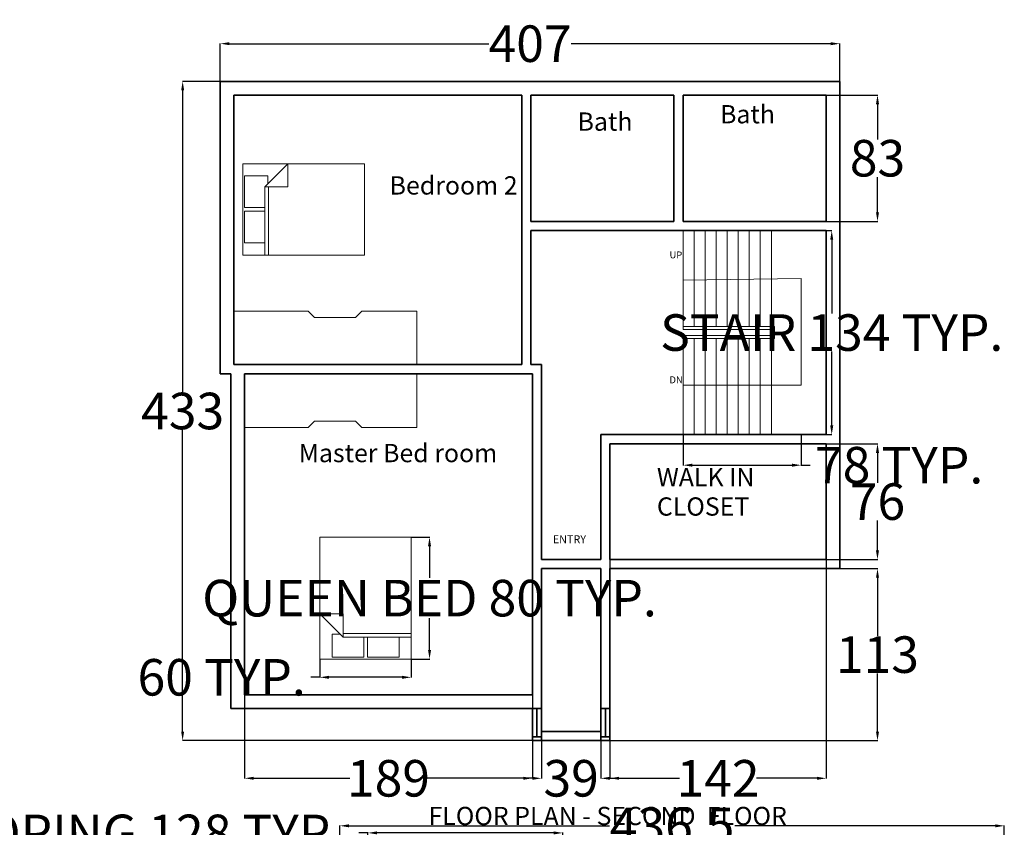
# Model space of a CAD drawing. Units: inches. Extents: x -15 to 1815, y 1023 to 2303.
# Tile 8 of 8: x 910 to 1556, y 1773 to 2303. Entities that reach past the tile are written whole.
import ezdxf

# ---------------------------------------------------------------- set-up
doc = ezdxf.new("R2010")
doc.units = ezdxf.units.IN
doc.header["$MEASUREMENT"] = 0
for name, color, linetype, lineweight in [('A-ANNO-DIMS', 2, 'Continuous', 18), ('A-ANNO-TEXT', 7, 'Continuous', 25), ('A-AREA-IDEN', 7, 'Continuous', 18), ('A-FLOR-STRS', 3, 'Continuous', 18), ('A-FURN', 8, 'Continuous', 18), ('A-WALL', 7, 'Continuous', 35)]:
    doc.layers.add(name, color=color, linetype=linetype, lineweight=lineweight)
doc.styles.get("Standard").update_dxf_attribs({"font": 'arial.ttf'})
doc.dimstyles.get("Standard").update_dxf_attribs({"dimtxt": 24, "dimasz": 6, "dimexe": 0.18, "dimexo": 0.0625, "dimgap": 0.09, "dimtad": 0, "dimtih": 1, "dimtoh": 1, "dimdec": 0, "dimzin": 0, "dimdsep": 46, "dimlunit": 3, "dimtxsty": 'Standard', "dimcen": 0.09, "dimadec": 0, "dimazin": 0, "dimtfac": 1, "dimtdec": 0, "dimtofl": 0, "dimtmove": 0, "dimatfit": 3, "dimfxl": 1, "dimtolj": 1, "dimtzin": 0, "dimarcsym": 0})

# ---------------------------------------------------------------- blocks, each defined once
blk = doc.blocks.new('Bed - Queen')
for p, q in [((0, -80.00003), (0, 0)), ((0, 0), (59.99999, 0)), ((59.99999, 0), (59.99999, -80.00003)), ((7.99999, -1.2), (28.79998, -1.2)), ((7.99999, -14.4), (7.99999, -1.2)), ((28.79998, -1.2), (28.79998, -14.4)), ((31.19999, -1.2), (51.99999, -1.2)), ((31.19999, -14.4), (31.19999, -1.2)), ((51.99999, -1.2), (51.99999, -16.4)), ((0, -14.4), (44.8, -14.4)), ((44.8, -16.8), (0, -16.8)), ((59.99999, -29.6), (44.8, -14.4)), ((44.8, -14.4), (44.8, -29.6)), ((51.99999, -16.4), (46.79936, -16.4)), ((44.8, -29.6), (59.99999, -29.6)), ((59.99999, -80.00003), (0, -80.00003))]:
    blk.add_line(p, q)
blk = doc.blocks.new('STAIR-RETURN-PLAN')
for p, q in [((0, 69), (0, 134)), ((7.25, 71), (7.25, 134)), ((14.5, 71), (14.5, 134)), ((21.75, 71), (21.75, 134)), ((29, 71), (29, 134)), ((36.25, 71), (36.25, 134)), ((43.5, 71), (43.5, 134)), ((50.75, 71), (50.75, 134)), ((58, 71), (58, 134)), ((58, 71), (58, 134)), ((0, 101.5), (77.56, 102.5)), ((77.56, 102.5), (77.56, 32.54)), ((60, 71), (0, 71)), ((58, 69), (0, 69)), ((58, 65), (0, 65)), ((0, 0), (0, 65)), ((58, 65), (58, 69)), ((60, 65), (60, 71)), ((60, 63), (60, 65)), ((60, 63), (0, 63)), ((7.25, 0), (7.25, 63)), ((14.5, 0), (14.5, 63)), ((21.75, 0), (21.75, 63)), ((29, 0), (29, 63)), ((36.25, 0), (36.25, 63)), ((43.5, 0), (43.5, 63)), ((50.75, 0), (50.75, 63)), ((58, 0), (58, 63)), ((58, 0), (58, 63)), ((77.56, 32.54), (0, 32.5))]:
    blk.add_line(p, q)
blk = doc.blocks.new('*D23')
at = {"layer": 'A-ANNO-DIMS', "color": 0, "lineweight": -2, "transparency": 16777216}
for p, q in [((1166.94, 1963.35), (1179.06, 1963.35)), ((1178.88, 1957.35), (1178.88, 1936.58)), ((1178.88, 1889.35), (1178.88, 1910.11)), ((1166.94, 1883.35), (1179.06, 1883.35))]:
    blk.add_line(p, q, dxfattribs=at)
at = {"layer": 'A-ANNO-DIMS', "color": 0, "transparency": 16777216}
for points in [[(1177.88, 1957.35), (1179.88, 1957.35), (1178.88, 1963.35)], [(1177.88, 1889.35), (1179.88, 1889.35), (1178.88, 1883.35)]]:
    blk.add_solid(points, dxfattribs=at)
at = {"layer": 'Defpoints', "color": 0, "transparency": 16777216}
for p in [(1166.88, 1963.35), (1166.88, 1883.35), (1178.88, 1883.35)]:
    blk.add_point(p, dxfattribs=at)
at = {"layer": 'A-ANNO-DIMS', "color": 0, "transparency": 16777216, "insert": (1178.88, 1923.35), "char_height": 24, "attachment_point": 5}
blk.add_mtext('\\A1;QUEEN BED 80 TYP.', dxfattribs=at)
blk = doc.blocks.new('*D24')
at = {"layer": 'A-ANNO-DIMS', "color": 0, "lineweight": -2, "transparency": 16777216}
for p, q in [((1106.88, 1883.29), (1106.88, 1871.17)), ((1166.88, 1883.29), (1166.88, 1871.17)), ((1106.88, 1871.35), (1100.88, 1871.35)), ((1160.88, 1871.35), (1112.88, 1871.35))]:
    blk.add_line(p, q, dxfattribs=at)
at = {"layer": 'A-ANNO-DIMS', "color": 0, "transparency": 16777216}
for points in [[(1112.88, 1872.35), (1112.88, 1870.35), (1106.88, 1871.35)], [(1160.88, 1872.35), (1160.88, 1870.35), (1166.88, 1871.35)]]:
    blk.add_solid(points, dxfattribs=at)
at = {"layer": 'Defpoints', "color": 0, "transparency": 16777216}
for p in [(1106.88, 1883.35), (1166.88, 1883.35), (1106.88, 1871.35)]:
    blk.add_point(p, dxfattribs=at)
at = {"layer": 'A-ANNO-DIMS', "color": 0, "transparency": 16777216, "insert": (1042.31, 1871.35), "char_height": 24, "attachment_point": 5}
blk.add_mtext('\\A1;60 TYP.', dxfattribs=at)
blk = doc.blocks.new('*D25')
at = {"layer": 'A-ANNO-DIMS', "color": 0, "lineweight": -2, "transparency": 16777216}
for p, q in [((1423.04, 2164.75), (1443.26, 2164.75)), ((1443.08, 2158.75), (1443.08, 2110.26)), ((1443.08, 2036.75), (1443.08, 2085.24)), ((1423.04, 2030.75), (1443.26, 2030.75))]:
    blk.add_line(p, q, dxfattribs=at)
at = {"layer": 'A-ANNO-DIMS', "color": 0, "transparency": 16777216}
for points in [[(1442.08, 2158.75), (1444.08, 2158.75), (1443.08, 2164.75)], [(1442.08, 2036.75), (1444.08, 2036.75), (1443.08, 2030.75)]]:
    blk.add_solid(points, dxfattribs=at)
at = {"layer": 'Defpoints', "color": 0, "transparency": 16777216}
for p in [(1422.98, 2164.75), (1443.08, 2164.75), (1422.98, 2030.75)]:
    blk.add_point(p, dxfattribs=at)
at = {"layer": 'A-ANNO-DIMS', "color": 0, "transparency": 16777216, "insert": (1443.08, 2097.75), "char_height": 24, "attachment_point": 5}
blk.add_mtext('\\A1;STAIR 134 TYP.', dxfattribs=at)
blk = doc.blocks.new('*D26')
at = {"layer": 'A-ANNO-DIMS', "color": 0, "lineweight": -2, "transparency": 16777216}
for p, q in [((1345.42, 2030.69), (1345.42, 2010.47)), ((1422.98, 2030.69), (1422.98, 2010.47)), ((1351.42, 2010.65), (1416.98, 2010.65)), ((1422.98, 2010.65), (1428.98, 2010.65))]:
    blk.add_line(p, q, dxfattribs=at)
at = {"layer": 'A-ANNO-DIMS', "color": 0, "transparency": 16777216}
for points in [[(1351.42, 2011.65), (1351.42, 2009.65), (1345.42, 2010.65)], [(1416.98, 2011.65), (1416.98, 2009.65), (1422.98, 2010.65)]]:
    blk.add_solid(points, dxfattribs=at)
at = {"layer": 'Defpoints', "color": 0, "transparency": 16777216}
for p in [(1345.42, 2030.75), (1422.98, 2030.75), (1422.98, 2010.65)]:
    blk.add_point(p, dxfattribs=at)
at = {"layer": 'A-ANNO-DIMS', "color": 0, "transparency": 16777216, "insert": (1487.38, 2010.65), "char_height": 24, "attachment_point": 5}
blk.add_mtext('\\A1;78 TYP.', dxfattribs=at)
blk = doc.blocks.new('*D45')
at = {"layer": 'A-ANNO-DIMS', "color": 0, "lineweight": -2, "transparency": 16777216}
for p, q in [((1138.43, 1769.16), (1132.43, 1769.16)), ((1138.43, 1750.02), (1138.43, 1769.34)), ((1260.44, 1769.16), (1144.43, 1769.16)), ((1266.44, 1750.02), (1266.44, 1769.34))]:
    blk.add_line(p, q, dxfattribs=at)
at = {"layer": 'A-ANNO-DIMS', "color": 0, "transparency": 16777216}
for points in [[(1144.43, 1770.16), (1144.43, 1768.16), (1138.43, 1769.16)], [(1260.44, 1770.16), (1260.44, 1768.16), (1266.44, 1769.16)]]:
    blk.add_solid(points, dxfattribs=at)
at = {"layer": 'Defpoints', "color": 0, "transparency": 16777216}
for p in [(1138.43, 1769.16), (1138.43, 1749.96), (1266.44, 1749.96)]:
    blk.add_point(p, dxfattribs=at)
at = {"layer": 'A-ANNO-DIMS', "color": 0, "transparency": 16777216, "insert": (993.96, 1769.16), "char_height": 24, "attachment_point": 5}
blk.add_mtext('\\A1;COPING 128 TYP.', dxfattribs=at)
blk = doc.blocks.new('*D80')
at = {"layer": 'A-ANNO-DIMS', "color": 0, "lineweight": -2, "transparency": 16777216}
for p, q in [((1041.42, 2262.81), (1041.42, 2287.66)), ((1047.42, 2287.48), (1217.83, 2287.48)), ((1442.42, 2287.48), (1272, 2287.48)), ((1448.42, 2262.81), (1448.42, 2287.66))]:
    blk.add_line(p, q, dxfattribs=at)
at = {"layer": 'A-ANNO-DIMS', "color": 0, "transparency": 16777216}
for points in [[(1047.42, 2288.48), (1047.42, 2286.48), (1041.42, 2287.48)], [(1442.42, 2288.48), (1442.42, 2286.48), (1448.42, 2287.48)]]:
    blk.add_solid(points, dxfattribs=at)
at = {"layer": 'Defpoints', "color": 0, "transparency": 16777216}
for p in [(1448.42, 2287.48), (1041.42, 2262.75), (1448.42, 2262.75)]:
    blk.add_point(p, dxfattribs=at)
at = {"layer": 'A-ANNO-DIMS', "color": 0, "transparency": 16777216, "insert": (1244.92, 2287.48), "char_height": 24, "attachment_point": 5}
blk.add_mtext('\\A1;407', dxfattribs=at)
blk = doc.blocks.new('*D81')
at = {"layer": 'A-ANNO-DIMS', "color": 0, "lineweight": -2, "transparency": 16777216}
for p, q in [((1041.36, 2262.75), (1016.51, 2262.75)), ((1016.69, 2256.75), (1016.69, 2058.6)), ((1016.69, 1835.75), (1016.69, 2033.9)), ((1246.36, 1829.75), (1016.51, 1829.75))]:
    blk.add_line(p, q, dxfattribs=at)
at = {"layer": 'A-ANNO-DIMS', "color": 0, "transparency": 16777216}
for points in [[(1015.69, 2256.75), (1017.69, 2256.75), (1016.69, 2262.75)], [(1015.69, 1835.75), (1017.69, 1835.75), (1016.69, 1829.75)]]:
    blk.add_solid(points, dxfattribs=at)
at = {"layer": 'Defpoints', "color": 0, "transparency": 16777216}
for p in [(1041.42, 2262.75), (1016.69, 1829.75), (1246.42, 1829.75)]:
    blk.add_point(p, dxfattribs=at)
at = {"layer": 'A-ANNO-DIMS', "color": 0, "transparency": 16777216, "insert": (1016.69, 2046.25), "char_height": 24, "attachment_point": 5}
blk.add_mtext('\\A1;433', dxfattribs=at)
blk = doc.blocks.new('*D82')
at = {"layer": 'A-ANNO-DIMS', "color": 0, "lineweight": -2, "transparency": 16777216}
for p, q in [((1448.48, 1942.75), (1473.33, 1942.75)), ((1473.15, 1936.75), (1473.15, 1898.6)), ((1473.15, 1835.75), (1473.15, 1873.9)), ((1297.48, 1829.75), (1473.33, 1829.75))]:
    blk.add_line(p, q, dxfattribs=at)
at = {"layer": 'A-ANNO-DIMS', "color": 0, "transparency": 16777216}
for points in [[(1472.15, 1936.75), (1474.15, 1936.75), (1473.15, 1942.75)], [(1472.15, 1835.75), (1474.15, 1835.75), (1473.15, 1829.75)]]:
    blk.add_solid(points, dxfattribs=at)
at = {"layer": 'Defpoints', "color": 0, "transparency": 16777216}
for p in [(1448.42, 1942.75), (1473.15, 1942.75), (1297.42, 1829.75)]:
    blk.add_point(p, dxfattribs=at)
at = {"layer": 'A-ANNO-DIMS', "color": 0, "transparency": 16777216, "insert": (1473.15, 1886.25), "char_height": 24, "attachment_point": 5}
blk.add_mtext('\\A1;113', dxfattribs=at)
blk = doc.blocks.new('*D83')
at = {"layer": 'A-ANNO-DIMS', "color": 0, "lineweight": -2, "transparency": 16777216}
for p, q in [((1439.48, 2024.75), (1473.33, 2024.75)), ((1473.15, 2018.75), (1473.15, 1999.09)), ((1473.15, 1954.75), (1473.15, 1974.41)), ((1439.48, 1948.75), (1473.33, 1948.75))]:
    blk.add_line(p, q, dxfattribs=at)
at = {"layer": 'A-ANNO-DIMS', "color": 0, "transparency": 16777216}
for points in [[(1472.15, 2018.75), (1474.15, 2018.75), (1473.15, 2024.75)], [(1472.15, 1954.75), (1474.15, 1954.75), (1473.15, 1948.75)]]:
    blk.add_solid(points, dxfattribs=at)
at = {"layer": 'Defpoints', "color": 0, "transparency": 16777216}
for p in [(1439.42, 2024.75), (1473.15, 2024.75), (1439.42, 1948.75)]:
    blk.add_point(p, dxfattribs=at)
at = {"layer": 'A-ANNO-DIMS', "color": 0, "transparency": 16777216, "insert": (1473.15, 1986.75), "char_height": 24, "attachment_point": 5}
blk.add_mtext('\\A1;76', dxfattribs=at)
blk = doc.blocks.new('*D84')
at = {"layer": 'A-ANNO-DIMS', "color": 0, "lineweight": -2, "transparency": 16777216}
for p, q in [((1439.48, 2253.75), (1473.33, 2253.75)), ((1473.15, 2247.75), (1473.15, 2224.6)), ((1473.15, 2176.75), (1473.15, 2199.9)), ((1439.48, 2170.75), (1473.33, 2170.75))]:
    blk.add_line(p, q, dxfattribs=at)
at = {"layer": 'A-ANNO-DIMS', "color": 0, "transparency": 16777216}
for points in [[(1472.15, 2247.75), (1474.15, 2247.75), (1473.15, 2253.75)], [(1472.15, 2176.75), (1474.15, 2176.75), (1473.15, 2170.75)]]:
    blk.add_solid(points, dxfattribs=at)
at = {"layer": 'Defpoints', "color": 0, "transparency": 16777216}
for p in [(1439.42, 2253.75), (1473.15, 2253.75), (1439.42, 2170.75)]:
    blk.add_point(p, dxfattribs=at)
at = {"layer": 'A-ANNO-DIMS', "color": 0, "transparency": 16777216, "insert": (1473.15, 2212.25), "char_height": 24, "attachment_point": 5}
blk.add_mtext('\\A1;83', dxfattribs=at)
blk = doc.blocks.new('*D85')
at = {"layer": 'A-ANNO-DIMS', "color": 0, "lineweight": -2, "transparency": 16777216}
for p, q in [((1057.42, 1859.69), (1057.42, 1804.84)), ((1246.42, 1859.69), (1246.42, 1804.84)), ((1063.42, 1805.02), (1126.42, 1805.02)), ((1240.42, 1805.02), (1177.42, 1805.02))]:
    blk.add_line(p, q, dxfattribs=at)
at = {"layer": 'A-ANNO-DIMS', "color": 0, "transparency": 16777216}
for points in [[(1063.42, 1806.02), (1063.42, 1804.02), (1057.42, 1805.02)], [(1240.42, 1806.02), (1240.42, 1804.02), (1246.42, 1805.02)]]:
    blk.add_solid(points, dxfattribs=at)
at = {"layer": 'Defpoints', "color": 0, "transparency": 16777216}
for p in [(1057.42, 1859.75), (1246.42, 1859.75), (1246.42, 1805.02)]:
    blk.add_point(p, dxfattribs=at)
at = {"layer": 'A-ANNO-DIMS', "color": 0, "transparency": 16777216, "insert": (1151.92, 1805.02), "char_height": 24, "attachment_point": 5}
blk.add_mtext('\\A1;189', dxfattribs=at)
blk = doc.blocks.new('*D86')
at = {"layer": 'A-ANNO-DIMS', "color": 0, "lineweight": -2, "transparency": 16777216}
for p, q in [((1252.417621, 1850.68843), (1252.417621, 1804.83843)), ((1291.417621, 1850.68843), (1291.417621, 1804.83843)), ((1246.417621, 1805.01843), (1240.417621, 1805.01843)), ((1297.417621, 1805.01843), (1303.417621, 1805.01843))]:
    blk.add_line(p, q, dxfattribs=at)
at = {"layer": 'A-ANNO-DIMS', "color": 0, "transparency": 16777216}
for points in [[(1246.417621, 1806.01843), (1246.417621, 1804.01843), (1252.417621, 1805.01843)], [(1297.417621, 1806.01843), (1297.417621, 1804.01843), (1291.417621, 1805.01843)]]:
    blk.add_solid(points, dxfattribs=at)
at = {"layer": 'Defpoints', "color": 0, "transparency": 16777216}
for p in [(1252.417621, 1850.75093), (1291.417621, 1850.75093), (1291.417621, 1805.01843)]:
    blk.add_point(p, dxfattribs=at)
at = {"layer": 'A-ANNO-DIMS', "color": 0, "transparency": 16777216, "insert": (1271.917621, 1805.01843), "char_height": 24, "attachment_point": 5}
blk.add_mtext('\\A1;39', dxfattribs=at)
blk = doc.blocks.new('*D87')
at = {"layer": 'A-ANNO-DIMS', "color": 0, "lineweight": -2, "transparency": 16777216}
for p, q in [((1297.42, 1948.69), (1297.42, 1804.84)), ((1439.42, 1948.69), (1439.42, 1804.84)), ((1303.42, 1805.02), (1343.07, 1805.02)), ((1433.42, 1805.02), (1393.77, 1805.02))]:
    blk.add_line(p, q, dxfattribs=at)
at = {"layer": 'A-ANNO-DIMS', "color": 0, "transparency": 16777216}
for points in [[(1303.42, 1806.02), (1303.42, 1804.02), (1297.42, 1805.02)], [(1433.42, 1806.02), (1433.42, 1804.02), (1439.42, 1805.02)]]:
    blk.add_solid(points, dxfattribs=at)
at = {"layer": 'Defpoints', "color": 0, "transparency": 16777216}
for p in [(1297.42, 1948.75), (1439.42, 1948.75), (1439.42, 1805.02)]:
    blk.add_point(p, dxfattribs=at)
at = {"layer": 'A-ANNO-DIMS', "color": 0, "transparency": 16777216, "insert": (1368.42, 1805.02), "char_height": 24, "attachment_point": 5}
blk.add_mtext('\\A1;142', dxfattribs=at)
blk = doc.blocks.new('*D103')
at = {"layer": 'A-ANNO-DIMS', "color": 0, "lineweight": -2, "transparency": 16777216}
for p, q in [((1119.96, 1657.14), (1119.96, 1773.99)), ((1125.96, 1773.81), (1297.05, 1773.81)), ((1550.46, 1773.81), (1379.37, 1773.81)), ((1556.46, 1657.14), (1556.46, 1773.99))]:
    blk.add_line(p, q, dxfattribs=at)
at = {"layer": 'A-ANNO-DIMS', "color": 0, "transparency": 16777216}
for points in [[(1125.96, 1774.81), (1125.96, 1772.81), (1119.96, 1773.81)], [(1550.46, 1774.81), (1550.46, 1772.81), (1556.46, 1773.81)]]:
    blk.add_solid(points, dxfattribs=at)
at = {"layer": 'Defpoints', "color": 0, "transparency": 16777216}
for p in [(1556.46, 1773.81), (1119.96, 1657.08), (1556.46, 1657.08)]:
    blk.add_point(p, dxfattribs=at)
at = {"layer": 'A-ANNO-DIMS', "color": 0, "transparency": 16777216, "insert": (1338.21, 1773.81), "char_height": 24, "attachment_point": 5}
blk.add_mtext('\\A1;436.5', dxfattribs=at)

msp = doc.modelspace()

# ---------------------------------------------------------------- linework, layer by layer
at = {"layer": 'A-FURN'}
for p, q in [((1050.4176, 2111.7493), (1099.1475, 2111.7493)), ((1099.1475, 2111.7493), (1103.3276, 2107.5692)), ((1130.2046, 2107.5692), (1134.3847, 2111.7493)), ((1134.3847, 2111.7493), (1170.5663, 2111.7493)), ((1170.5663, 2111.7493), (1170.5663, 2076.7509)), ((1103.3276, 2107.5692), (1130.2046, 2107.5692)), ((1170.5663, 2035.4596), (1170.5663, 2070.458)), ((1099.1475, 2035.4596), (1103.3276, 2039.6397)), ((1103.3276, 2039.6397), (1130.2046, 2039.6397)), ((1130.2046, 2039.6397), (1134.3847, 2035.4596)), ((1057.4176, 2035.4596), (1099.1475, 2035.4596)), ((1134.3847, 2035.4596), (1170.5663, 2035.4596))]:
    msp.add_line(p, q, dxfattribs=at)
at = {"layer": 'A-WALL'}
for p, q in [((1041.4176, 2070.7509), (1041.4176, 2262.7509)), ((1041.4176, 2262.7509), (1448.4176, 2262.7509)), ((1245.4176, 2262.7509), (1339.4176, 2262.7509)), ((1345.4176, 2262.7509), (1439.4176, 2262.7509)), ((1448.4176, 2262.7509), (1448.4176, 2170.7509)), ((1448.4176, 2262.7509), (1448.4176, 2030.7509)), ((1448.4176, 2262.7509), (1448.4176, 1942.7509)), ((1050.4176, 2253.7509), (1239.4176, 2253.7509)), ((1050.4176, 2076.7509), (1050.4176, 2253.7509)), ((1239.4176, 2253.7509), (1239.4176, 2076.7509)), ((1245.4176, 2253.7509), (1245.4176, 2170.7509)), ((1245.4176, 2253.7509), (1339.4176, 2253.7509)), ((1339.4176, 2253.7509), (1339.4176, 2170.7509)), ((1345.4176, 2253.7509), (1345.4176, 2170.7509)), ((1345.4176, 2253.7509), (1439.4176, 2253.7509)), ((1439.4176, 2253.7509), (1439.4176, 2170.7509)), ((1339.4176, 2170.7509), (1245.4176, 2170.7509)), ((1439.4176, 2170.7509), (1345.4176, 2170.7509)), ((1339.4176, 2164.7509), (1245.4176, 2164.7509)), ((1439.4176, 2164.7509), (1245.4176, 2164.7509)), ((1245.4176, 2164.7509), (1245.4176, 2076.7509)), ((1439.4176, 2164.7509), (1439.4176, 2030.7509)), ((1239.4176, 2076.7509), (1050.4176, 2076.7509)), ((1252.4176, 2076.7509), (1245.4176, 2076.7509)), ((1252.4176, 1948.7509), (1252.4176, 2076.7509)), ((1048.4176, 2070.7509), (1041.4176, 2070.7509)), ((1048.4176, 1850.7509), (1048.4176, 2070.7509)), ((1246.4176, 2070.7509), (1057.4176, 2070.7509)), ((1057.4176, 1859.7509), (1057.4176, 2070.7509)), ((1246.4176, 1859.7509), (1246.4176, 2070.7509)), ((1439.4176, 2030.7509), (1291.4176, 2030.7509)), ((1291.4176, 1948.7509), (1291.4176, 2030.7509)), ((1439.4176, 2024.7509), (1297.4176, 2024.7509)), ((1297.4176, 1948.7509), (1297.4176, 2024.7509)), ((1439.4176, 2024.7509), (1439.4176, 1948.7509)), ((1291.4176, 1948.7509), (1252.4176, 1948.7509)), ((1439.4176, 1948.7509), (1297.4176, 1948.7509)), ((1252.4176, 1835.7509), (1252.4176, 1942.7509)), ((1291.4176, 1942.7509), (1252.4176, 1942.7509)), ((1291.4176, 1835.7509), (1291.4176, 1942.7509)), ((1448.4176, 1942.7509), (1297.4176, 1942.7509)), ((1297.4176, 1850.7509), (1297.4176, 1942.7509)), ((1246.4176, 1859.7509), (1057.4176, 1859.7509)), ((1246.4176, 1850.7509), (1048.4176, 1850.7509)), ((1246.4176, 1829.7509), (1246.4176, 1850.7509)), ((1252.4176, 1850.7509), (1246.4176, 1850.7509)), ((1249.4176, 1850.7509), (1249.4176, 1832.2066)), ((1297.4176, 1850.7509), (1291.4176, 1850.7509)), ((1297.4176, 1850.7509), (1291.4176, 1850.7509)), ((1291.4176, 1850.7509), (1294.4176, 1850.7509)), ((1294.4176, 1850.7509), (1294.4176, 1832.2066)), ((1297.4176, 1829.7509), (1297.4176, 1850.7509)), ((1252.4176, 1832.2066), (1246.4176, 1832.2066)), ((1291.4176, 1835.7509), (1252.4176, 1835.7509)), ((1252.4176, 1835.7509), (1252.4176, 1829.7509)), ((1291.4176, 1835.7509), (1291.4176, 1829.7509)), ((1297.4176, 1832.2066), (1291.4176, 1832.2066)), ((1297.4176, 1829.7509), (1246.4176, 1829.7509))]:
    msp.add_line(p, q, dxfattribs=at)

# ---------------------------------------------------------------- block references
at = {"layer": 'A-FLOR-STRS'}
msp.add_blockref('STAIR-RETURN-PLAN', (1345.4176, 2030.7509), dxfattribs=at)
at = {"layer": 'A-FURN'}
for p, rotation in [((1056.2068, 2148.589), 89.99999999999999), ((1166.8819, 1883.349), 180)]:
    msp.add_blockref('Bed - Queen', p, dxfattribs=dict(at, rotation=rotation))

# ---------------------------------------------------------------- texts
at = {"layer": 'A-ANNO-TEXT'}
for s, height, p in [('UP', 4.53138, (1336.5144, 2146.474)), ('DN', 4.53138, (1336.5144, 2064.4435)), ('FLOOR PLAN - SECOND  FLOOR', 12, (1178.2311, 1774.2654))]:
    msp.add_text(s, height=height, dxfattribs=at).set_placement(p)
at = {"layer": 'A-AREA-IDEN'}
for s, height, p in [('Bath', 12, (1369.7329, 2235.1609)), ('Bath', 12, (1276.1186, 2230.323)), ('Bedroom 2', 12, (1152.6446, 2188.394)), ('Master Bed room', 12, (1092.9251, 2012.615)), ('WALK IN ', 12, (1328.2482, 1996.7945)), ('CLOSET', 12, (1328.2482, 1977.5176)), ('ENTRY', 5.21216, (1259.8202, 1959.399))]:
    msp.add_text(s, height=height, dxfattribs=at).set_placement(p)

# ---------------------------------------------------------------- dimensions: what is measured, and where the dimension line sits
at = {"layer": 'A-ANNO-DIMS'}
for base, p1, p2, override, picture, middle in [((1448.4176, 2287.4834), (1041.4176, 2262.7509), (1448.4176, 2262.7509), {"dimdec": 0, "dimlfac": 1, "dimrnd": 0, "dimzin": 0, "dimdsep": 46, "dimlunit": 2}, '*D80', (1244.9176, 2287.4834)), ((1439.4176, 1805.0184), (1297.4176, 1948.7509), (1439.4176, 1948.7509), {"dimdec": 0, "dimlfac": 1, "dimrnd": 0, "dimzin": 0, "dimdsep": 46, "dimlunit": 2}, '*D87', (1368.4176, 1805.0184)), ((1246.4176, 1805.0184), (1057.4176, 1859.7509), (1246.4176, 1859.7509), {"dimdec": 0, "dimlfac": 1, "dimrnd": 0, "dimzin": 0, "dimdsep": 46, "dimlunit": 2}, '*D85', (1151.9176, 1805.0184)), ((1291.4176, 1805.0184), (1252.4176, 1850.7509), (1291.4176, 1850.7509), {"dimdec": 0, "dimlfac": 1, "dimrnd": 0, "dimzin": 0, "dimdsep": 46, "dimlunit": 2}, '*D86', (1271.9176, 1805.0184)), ((1556.4613, 1773.8085), (1119.956, 1657.0773), (1556.4613, 1657.0773), {"dimdec": 1, "dimlfac": 1, "dimrnd": 0, "dimzin": 0, "dimdsep": 46, "dimlunit": 2}, '*D103', (1338.2086, 1773.8085))]:
    dim = msp.add_linear_dim(base=base, p1=p1, p2=p2, dimstyle='Standard', override=override, dxfattribs=at)
    dim.commit()
    dim.dimension.update_dxf_attribs({"geometry": picture, "text_midpoint": middle})
for base, p1, p2, picture, middle in [((1016.6851, 1829.7509), (1041.4176, 2262.7509), (1246.4176, 1829.7509), '*D81', (1016.6851, 2046.2509)), ((1473.1501, 2253.7509), (1439.4176, 2170.7509), (1439.4176, 2253.7509), '*D84', (1473.1501, 2212.2509)), ((1473.1501, 2024.7509), (1439.4176, 1948.7509), (1439.4176, 2024.7509), '*D83', (1473.1501, 1986.7509)), ((1473.1501, 1942.7509), (1297.4176, 1829.7509), (1448.4176, 1942.7509), '*D82', (1473.1501, 1886.2509))]:
    dim = msp.add_linear_dim(base=base, p1=p1, p2=p2, angle=90, dimstyle='Standard', override={"dimdec": 0, "dimlfac": 1, "dimrnd": 0, "dimzin": 0, "dimdsep": 46, "dimlunit": 2}, dxfattribs=at)
    dim.commit()
    dim.dimension.update_dxf_attribs({"geometry": picture, "text_midpoint": middle})
for base, p1, p2, angle, text, picture, middle in [((1443.0789, 2164.7509), (1422.9789, 2030.7509), (1422.9789, 2164.7509), 90, 'STAIR <> TYP.', '*D25', (1443.0789, 2097.7509)), ((1178.8819, 1883.349), (1166.8819, 1963.349), (1166.8819, 1883.349), 270, 'QUEEN BED <> TYP.', '*D23', (1178.8819, 1923.349)), ((1106.8819, 1871.349), (1166.8819, 1883.349), (1106.8819, 1883.349), 180, '<> TYP.', '*D24', (1042.3144, 1871.349)), ((1138.4338, 1769.1591), (1266.4376, 1749.9585), (1138.4338, 1749.9585), 180, 'COPING <> TYP.', '*D45', (993.9591, 1769.1591))]:
    dim = msp.add_linear_dim(base=base, p1=p1, p2=p2, angle=angle, text=text, dimstyle='Standard', override={"dimdec": 0, "dimlfac": 1, "dimrnd": 0, "dimzin": 0, "dimdsep": 46, "dimlunit": 2}, dxfattribs=at)
    dim.commit()
    dim.dimension.update_dxf_attribs({"geometry": picture, "text_midpoint": middle})
dim = msp.add_linear_dim(base=(1422.9789, 2010.6509), p1=(1345.4176, 2030.7509), p2=(1422.9789, 2030.7509), text='<> TYP.', dimstyle='Standard', override={"dimdec": 0, "dimlfac": 1, "dimrnd": 0, "dimzin": 0, "dimdsep": 46, "dimlunit": 2}, dxfattribs=at)
dim.commit()
dim.dimension.update_dxf_attribs({"geometry": '*D26', "text_midpoint": (1487.3827, 2010.6509)})

doc.saveas('drawing.dxf')
